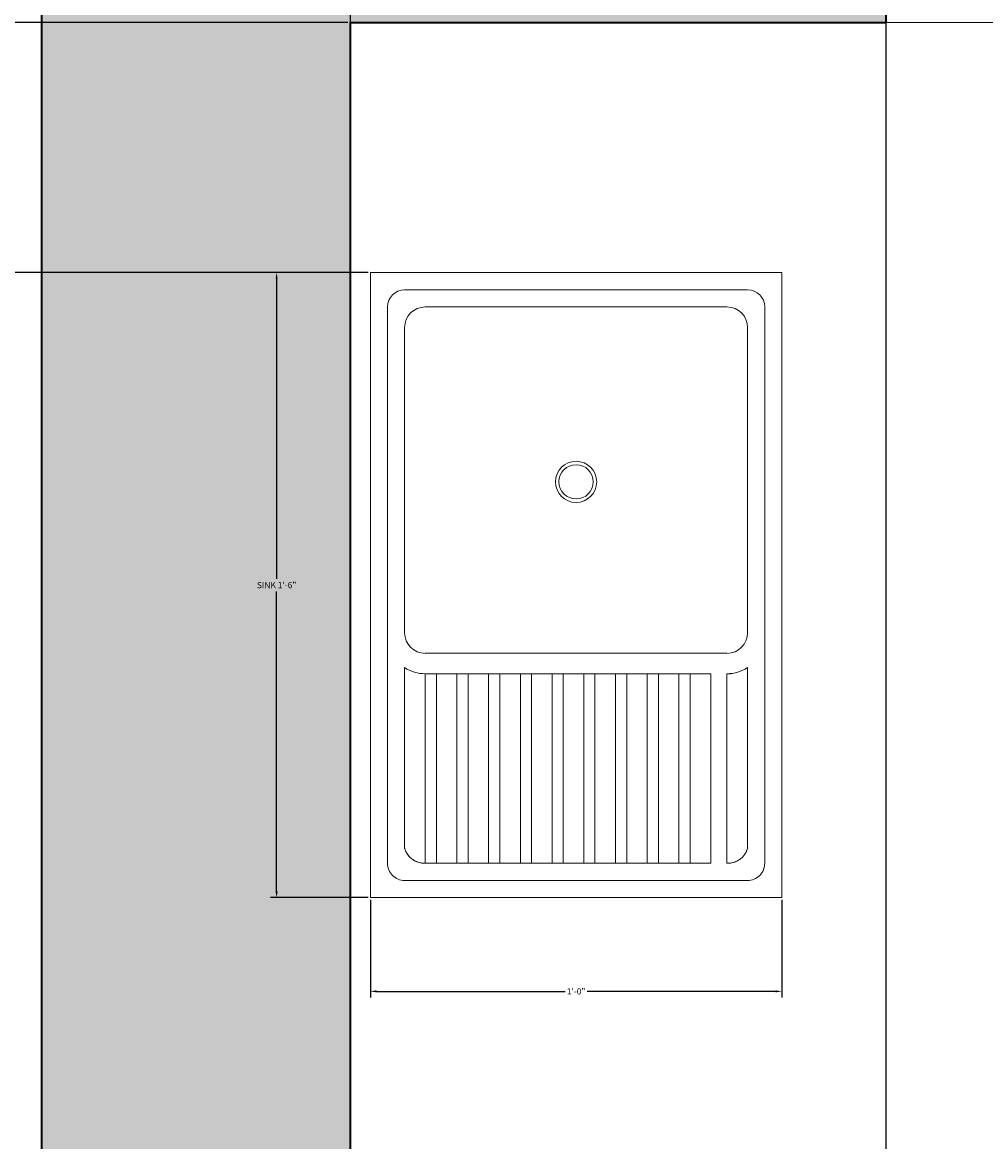
# Model space of a CAD drawing. Units: inches. Extents: x -5 to 330, y -522 to 40.
# Tile 10 of 23: x 23 to 51, y -330 to -297. Entities that reach past the tile are written whole.
import ezdxf

# ---------------------------------------------------------------- set-up
doc = ezdxf.new("R2010")
doc.units = ezdxf.units.IN
doc.header["$MEASUREMENT"] = 0
doc.linetypes.add('ACAD_ISO02W100', pattern=[15, 12, -3])
for name, color, linetype, lineweight in [('A-ANNO-DIMS', 2, 'Continuous', 18), ('A-FLOR-CASE', 8, 'Continuous', 25), ('A-FLOR-FIXT', 8, 'Continuous', 18), ('A-WALL', 7, 'Continuous', 35), ('A-WALL-OVHD', 8, 'ACAD_ISO02W100', 18)]:
    doc.layers.add(name, color=color, linetype=linetype, lineweight=lineweight)
doc.layers.add('A-WALL-PATT', color=18, linetype='Continuous', lineweight=13, true_color=0x000000)
doc.styles.get("Standard").update_dxf_attribs({"font": 'arial.ttf'})
doc.dimstyles.get("Standard").update_dxf_attribs({"dimtxt": 0.18, "dimasz": 0.18, "dimexe": 0.18, "dimexo": 0.0625, "dimgap": 0.09, "dimtad": 0, "dimtih": 1, "dimtoh": 1, "dimdec": 0, "dimzin": 0, "dimdsep": 46, "dimlunit": 3, "dimtxsty": 'Standard', "dimcen": 0.09, "dimadec": 0, "dimazin": 0, "dimtfac": 1, "dimtdec": 0, "dimtofl": 0, "dimtmove": 0, "dimatfit": 3, "dimfxl": 1, "dimtolj": 1, "dimtzin": 0, "dimarcsym": 0})

# ---------------------------------------------------------------- blocks, each defined once
blk = doc.blocks.new('*D2')
at = {"layer": 'A-ANNO-DIMS', "color": 0, "lineweight": -2, "transparency": 16777216}
for p, q in [((23.447, 12.356), (6.274, 12.356)), ((6.454, 12.176), (6.454, -203.738)), ((6.454, -425.964), (6.454, -210.049)), ((23.447, -426.144), (6.274, -426.144))]:
    blk.add_line(p, q, dxfattribs=at)
at = {"layer": 'A-ANNO-DIMS', "color": 0, "transparency": 16777216}
for points in [[(6.424, 12.176), (6.484, 12.176), (6.454, 12.356)], [(6.424, -425.964), (6.484, -425.964), (6.454, -426.144)]]:
    blk.add_solid(points, dxfattribs=at)
at = {"layer": 'Defpoints', "color": 0, "transparency": 16777216}
for p in [(23.51, 12.356), (6.454, -426.144), (23.51, -426.144)]:
    blk.add_point(p, dxfattribs=at)
at = {"layer": 'A-ANNO-DIMS', "color": 0, "transparency": 16777216, "insert": (6.454, -206.894), "char_height": 6, "attachment_point": 5}
blk.add_mtext('\\A1;36\'-7"', dxfattribs=at)
blk = doc.blocks.new('М12 540х820')
for p, q in [((0, 540), (-820, 540)), ((-820, 540), (-820, 0)), ((0, 0), (0, 540)), ((-45, 517.5), (-775, 517.5)), ((-797.5, 495), (-797.5, 45)), ((-347.5, 495), (-748, 495)), ((-301.7, 495), (-64.8, 495)), ((-22.5, 45), (-22.5, 495)), ((-293.7, 468), (-293.7, 472.5)), ((-775, 468), (-775, 72)), ((-320.5, 468), (-320.5, 72)), ((-293.7, 468), (-45, 468)), ((-45, 469.5), (-45, 468)), ((-293.7, 446.6), (-45, 446.6)), ((-293.7, 419.6), (-293.7, 446.6)), ((-45, 419.6), (-45, 446.6)), ((-293.7, 419.6), (-45, 419.6)), ((-293.7, 405), (-45, 405)), ((-293.7, 378), (-293.7, 405)), ((-45, 378), (-45, 405)), ((-293.7, 378), (-45, 378)), ((-293.7, 336.4), (-293.7, 363.4)), ((-293.7, 363.4), (-45, 363.4)), ((-45, 336.4), (-45, 363.4)), ((-293.7, 336.4), (-45, 336.4)), ((-293.7, 294.7), (-293.7, 321.7)), ((-293.7, 321.7), (-45, 321.7)), ((-45, 294.7), (-45, 321.7)), ((-293.7, 294.7), (-45, 294.7)), ((-293.7, 253.1), (-293.7, 280.1)), ((-293.7, 280.1), (-45, 280.1)), ((-45, 253.1), (-45, 280.1)), ((-293.7, 253.1), (-45, 253.1)), ((-293.7, 211.5), (-293.7, 238.5)), ((-293.7, 238.5), (-45, 238.5)), ((-45, 211.5), (-45, 238.5)), ((-293.7, 211.5), (-45, 211.5)), ((-293.7, 169.9), (-293.7, 196.9)), ((-293.7, 196.9), (-45, 196.9)), ((-45, 169.9), (-45, 196.9)), ((-293.7, 169.9), (-45, 169.9)), ((-293.7, 128.2), (-293.7, 155.2)), ((-293.7, 155.2), (-45, 155.2)), ((-45, 128.2), (-45, 155.2)), ((-293.7, 128.2), (-45, 128.2)), ((-293.7, 113.6), (-45, 113.6)), ((-293.7, 86.6), (-293.7, 113.6)), ((-45, 86.6), (-45, 113.6)), ((-293.7, 86.6), (-45, 86.6)), ((-293.7, 72), (-45, 72)), ((-45, 70.5), (-45, 72)), ((-748, 45), (-347.5, 45)), ((-301.7, 45), (-64.8, 45)), ((-775, 22.5), (-45, 22.5)), ((-820, 0), (0, 0))]:
    blk.add_line(p, q)
at = {"ltscale": 0.06}
for p, q in [((-820, 0), (-820, 540)), ((-820, 540), (0, 540)), ((0, 540), (0, 536.9)), ((0, 536.9), (0, 0)), ((-293.7, 446.6), (-45, 446.6)), ((-293.7, 405), (-293.7, 446.6)), ((-45, 446.6), (-45, 419.6)), ((-45, 419.6), (-45, 378)), ((-293.7, 363.4), (-293.7, 405)), ((-45, 378), (-45, 336.4)), ((-293.7, 321.7), (-293.7, 363.4)), ((-45, 336.4), (-45, 294.7)), ((-293.7, 280.1), (-293.7, 321.7)), ((-45, 294.7), (-45, 253.1)), ((-293.7, 238.5), (-293.7, 280.1)), ((-45, 253.1), (-45, 211.5)), ((-293.7, 196.9), (-293.7, 238.5)), ((-45, 211.5), (-45, 169.9)), ((-293.7, 155.2), (-293.7, 196.9)), ((-45, 169.9), (-45, 128.2)), ((-293.7, 113.6), (-293.7, 155.2)), ((-45, 128.2), (-45, 86.6)), ((-293.7, 72), (-293.7, 113.6)), ((-45, 86.6), (-45, 72)), ((-45, 72), (-293.7, 72)), ((0, 0), (-820, 0))]:
    blk.add_line(p, q, dxfattribs=at)
at = {"extrusion": (0, 0, -1)}
for centre, major_axis, start_param, end_param in [((-775, 495), (-15.9, 15.9), -0.785398, 0.785398), ((-775, 495), (-15.9, 15.9), -0.785398, 0.785398), ((-45, 495), (-15.9, -15.9), 2.356194, 3.926991), ((-45, 495), (-15.9, -15.9), 2.356194, 3.926991), ((-748, 468), (-19.1, -19.1), 0.785398, 2.356194), ((-748, 468), (-19.1, -19.1), 0.785398, 2.356194), ((-347.5, 468), (-19.1, 19.1), 0.785398, 2.356194), ((-347.5, 468), (-19.1, 19.1), 0.785398, 2.356194), ((-343.2, 468), (-35, 35), 1.779263, 2.356194), ((-343.2, 468), (-35, 35), 1.779263, 2.356192), ((-72.3, 468.8), (-19.3, 19.3), 1.0328, 2.38382), ((-72.3, 468.8), (-19.3, 19.3), 1.0328, 1.064673), ((-72.3, 468.8), (-19.3, 19.3), 1.064673, 2.328569), ((-343.2, 468), (-35, 35), 2.356192, 2.356194), ((-72.3, 468.8), (-19.3, 19.3), 2.328569, 2.38382), ((-545.5, 270), (-19.1, -19.1), 3.926991, 10.210176), ((-545.5, 270), (-19.1, -19.1), 3.926991, 10.210176), ((-545.5, 270), (-15.9, -15.9), 3.926991, 10.210176), ((-545.5, 270), (-15.9, -15.9), 3.926991, 10.210176), ((-748, 72), (-19.1, 19.1), 3.926991, 5.497787), ((-748, 72), (-19.1, 19.1), 3.926991, 5.497787), ((-347.5, 72), (-19.1, -19.1), 3.926991, 5.497787), ((-347.5, 72), (-19.1, -19.1), 3.926991, 5.497787), ((-343.2, 72), (-35, -35), 3.926991, 4.503922), ((-343.2, 72), (-35, -35), 3.926991, 4.503922), ((-72.3, 71.2), (-19.3, -19.3), 3.899365, 5.250385), ((-72.3, 71.2), (-19.3, -19.3), 3.954617, 5.218512), ((-72.3, 71.2), (-19.3, -19.3), 3.899365, 3.954617), ((-775, 45), (-15.9, -15.9), 5.497787, 7.068583), ((-775, 45), (-15.9, -15.9), 5.497787, 7.068583), ((-72.3, 71.2), (-19.3, -19.3), 5.218512, 5.250385), ((-45, 45), (-15.9, 15.9), 2.356194, 3.926991), ((-45, 45), (-15.9, 15.9), 2.356194, 3.926991)]:
    blk.add_ellipse(centre, major_axis=major_axis, ratio=1, start_param=start_param, end_param=end_param, dxfattribs=at)
blk = doc.blocks.new('*D33')
at = {"layer": 'A-ANNO-DIMS', "color": 0, "lineweight": -2, "transparency": 16777216}
for p, q in [((33.036, -304.441), (30.185, -304.441)), ((30.365, -304.621), (30.365, -313.37)), ((30.365, -322.485), (30.365, -313.736)), ((33.036, -322.665), (30.185, -322.665))]:
    blk.add_line(p, q, dxfattribs=at)
at = {"layer": 'A-ANNO-DIMS', "color": 0, "transparency": 16777216}
for points in [[(30.335, -304.621), (30.395, -304.621), (30.365, -304.441)], [(30.335, -322.485), (30.395, -322.485), (30.365, -322.665)]]:
    blk.add_solid(points, dxfattribs=at)
at = {"layer": 'Defpoints', "color": 0, "transparency": 16777216}
for p in [(33.099, -304.441), (30.365, -322.665), (33.099, -322.665)]:
    blk.add_point(p, dxfattribs=at)
at = {"layer": 'A-ANNO-DIMS', "color": 0, "transparency": 16777216, "insert": (30.365, -313.553), "char_height": 0.18, "attachment_point": 5}
blk.add_mtext('\\A1;SINK 1\'-6"', dxfattribs=at)
blk = doc.blocks.new('*D34')
at = {"layer": 'A-ANNO-DIMS', "color": 0, "lineweight": -2, "transparency": 16777216}
for p, q in [((33.099, -322.728), (33.099, -325.579)), ((45.1, -322.728), (45.1, -325.579)), ((33.279, -325.399), (38.778, -325.399)), ((44.92, -325.399), (39.42, -325.399))]:
    blk.add_line(p, q, dxfattribs=at)
at = {"layer": 'A-ANNO-DIMS', "color": 0, "transparency": 16777216}
for points in [[(33.279, -325.369), (33.279, -325.429), (33.099, -325.399)], [(44.92, -325.369), (44.92, -325.429), (45.1, -325.399)]]:
    blk.add_solid(points, dxfattribs=at)
at = {"layer": 'Defpoints', "color": 0, "transparency": 16777216}
for p in [(33.099, -322.665), (45.1, -322.665), (45.1, -325.399)]:
    blk.add_point(p, dxfattribs=at)
at = {"layer": 'A-ANNO-DIMS', "color": 0, "transparency": 16777216, "insert": (39.099, -325.399), "char_height": 0.18, "attachment_point": 5}
blk.add_mtext('\\A1;1\'-0"', dxfattribs=at)
blk = doc.blocks.new('*D40')
at = {"layer": 'A-ANNO-DIMS', "color": 0, "lineweight": -2, "transparency": 16777216}
for p, q in [((32.51, -246.706), (32.51, -522.309)), ((79.01, -246.706), (79.01, -522.309)), ((32.69, -522.129), (55.151, -522.129)), ((78.83, -522.129), (56.369, -522.129))]:
    blk.add_line(p, q, dxfattribs=at)
at = {"layer": 'A-ANNO-DIMS', "color": 0, "transparency": 16777216}
for points in [[(32.69, -522.099), (32.69, -522.159), (32.51, -522.129)], [(78.83, -522.099), (78.83, -522.159), (79.01, -522.129)]]:
    blk.add_solid(points, dxfattribs=at)
at = {"layer": 'Defpoints', "color": 0, "transparency": 16777216}
for p in [(32.51, -246.644), (79.01, -246.644), (79.01, -522.129)]:
    blk.add_point(p, dxfattribs=at)
at = {"layer": 'A-ANNO-DIMS', "color": 0, "transparency": 16777216, "insert": (55.76, -522.129), "char_height": 0.18, "attachment_point": 5}
blk.add_mtext('\\A1;3\'-10 1/2"', dxfattribs=at)
blk = doc.blocks.new('*D47')
at = {"layer": 'A-ANNO-DIMS', "color": 0, "lineweight": -2, "transparency": 16777216}
for p, q in [((32.447, -297.144), (-3.655, -297.144)), ((-3.475, -297.324), (-3.475, -300.609)), ((-3.475, -304.261), (-3.475, -300.975)), ((33.036, -304.441), (-3.655, -304.441))]:
    blk.add_line(p, q, dxfattribs=at)
at = {"layer": 'A-ANNO-DIMS', "color": 0, "transparency": 16777216}
for points in [[(-3.505, -297.324), (-3.445, -297.324), (-3.475, -297.144)], [(-3.505, -304.261), (-3.445, -304.261), (-3.475, -304.441)]]:
    blk.add_solid(points, dxfattribs=at)
at = {"layer": 'Defpoints', "color": 0, "transparency": 16777216}
for p in [(32.51, -297.144), (-3.475, -304.441), (33.099, -304.441)]:
    blk.add_point(p, dxfattribs=at)
at = {"layer": 'A-ANNO-DIMS', "color": 0, "transparency": 16777216, "insert": (-3.475, -300.792), "char_height": 0.18, "attachment_point": 5}
blk.add_mtext('\\A1;0\'-7 1/2"', dxfattribs=at)

msp = doc.modelspace()

# ---------------------------------------------------------------- hatches: boundary and pattern name
at = {"layer": 'A-WALL-PATT'}
h = msp.add_hatch(color=256, dxfattribs=at)
h.dxf.hatch_style = 1
h.paths.add_polyline_path([(164.01, -44.152), (159.51, -44.152), (159.51, -153.144), (164.01, -153.144)], flags=17)
h.paths.add_polyline_path([(224.01, -188.144), (272.01, -188.144), (272.01, -218.144), (260.01, -218.144), (260.01, -222.644), (272.01, -222.644), (272.01, -292.644), (159.01, -292.644), (159.01, -297.144), (272.01, -297.144), (272.01, -417.144), (245.51, -417.144), (245.51, -426.144), (272.01, -426.144), (272.01, -495.144), (281.01, -495.144), (281.01, 12.356), (23.51, 12.356), (23.51, -426.144), (62.918, -426.144), (62.918, -417.144), (32.51, -417.144), (32.51, -297.144), (48.129, -297.144), (48.129, -292.644), (32.51, -292.644), (32.51, -140.644), (133.51, -140.644), (133.51, -131.644), (32.51, -131.644), (32.51, 3.356), (159.51, 3.356), (164.01, 3.356), (220.01, 3.356), (224.51, 3.356), (272.01, 3.356), (272.01, -179.144), (159.51, -179.144), (159.51, -188.144), (219.51, -188.144), (219.51, -266.644), (224.01, -266.644), (224.01, -222.644), (236.01, -222.644), (236.01, -218.144), (224.01, -218.144)])
h.paths.add_polyline_path([(133.01, -292.644), (128.51, -292.644), (128.51, -297.144), (128.51, -417.144), (122.918, -417.144), (122.918, -426.144), (133.01, -426.144)], flags=17)
h.paths.add_polyline_path([(185.51, -417.144), (159.01, -417.144), (159.01, -426.144), (185.51, -426.144)], flags=17)
h.paths.add_polyline_path([(133.51, -140.644), (129.01, -140.644), (129.01, -246.644), (133.51, -246.644)], flags=17)
h.paths.add_polyline_path([(246.01, -48.644), (224.51, -48.644), (224.51, -27.627), (220.01, -27.627), (220.01, -48.644), (198.604, -48.644), (198.604, -53.144), (246.01, -53.144)], flags=17)

# ---------------------------------------------------------------- linework, layer by layer
at = {"layer": 'A-FLOR-CASE'}
msp.add_line((48.129, -297.144), (48.129, -393.928), dxfattribs=at)
at = {"layer": 'A-WALL'}
for p, q in [((23.51, 12.356), (23.51, -495.144)), ((48.129, -292.644), (48.129, -297.144)), ((32.51, -297.144), (48.129, -297.144)), ((32.51, -297.144), (32.51, -417.144))]:
    msp.add_line(p, q, dxfattribs=at)
at = {"layer": 'A-WALL-OVHD'}
msp.add_line((48.129, -297.144), (128.51, -297.144), dxfattribs=at)

# ---------------------------------------------------------------- block references
at = {"layer": 'A-FLOR-FIXT', "xscale": 0.0222246795123264, "yscale": 0.0222246795123264, "zscale": 0.0222246795123264, "rotation": 270}
msp.add_blockref('М12 540х820', (33.099, -322.665), dxfattribs=at)

# ---------------------------------------------------------------- dimensions: what is measured, and where the dimension line sits
at = {"layer": 'A-ANNO-DIMS'}
for base, p1, p2, override, picture, middle in [((6.454321893, -426.143582029), (23.509888577, 12.356417971), (23.509888577, -426.143582029), {"dimtxt": 6, "dimclrd": 0, "dimclre": 0, "dimclrt": 0}, '*D2', (6.454321893, -206.893582029)), ((-3.475, -304.441), (32.51, -297.144), (33.099, -304.441), {"dimdec": 1, "dimlfac": 1, "dimrnd": 0, "dimzin": 1, "dimdsep": 46, "dimlunit": 4, "dimfrac": 2}, '*D47', (-3.475, -300.792))]:
    dim = msp.add_linear_dim(base=base, p1=p1, p2=p2, angle=90, dimstyle='Standard', override=override, dxfattribs=at)
    dim.commit()
    dim.dimension.update_dxf_attribs({"geometry": picture, "text_midpoint": middle})
for base, p1, p2, picture, middle in [((79.01, -522.129), (32.51, -246.644), (79.01, -246.644), '*D40', (55.76, -522.129)), ((45.1, -325.399), (33.099, -322.665), (45.1, -322.665), '*D34', (39.099, -325.399))]:
    dim = msp.add_linear_dim(base=base, p1=p1, p2=p2, dimstyle='Standard', override={"dimdec": 1, "dimlfac": 1, "dimrnd": 0, "dimzin": 1, "dimdsep": 46, "dimlunit": 4, "dimfrac": 2}, dxfattribs=at)
    dim.commit()
    dim.dimension.update_dxf_attribs({"geometry": picture, "text_midpoint": middle})
dim = msp.add_linear_dim(base=(30.365, -322.665), p1=(33.099, -304.441), p2=(33.099, -322.665), angle=270, text='SINK <>', dimstyle='Standard', override={"dimdec": 1, "dimlfac": 1, "dimrnd": 0, "dimzin": 1, "dimdsep": 46, "dimlunit": 4, "dimfrac": 2}, dxfattribs=at)
dim.commit()
dim.dimension.update_dxf_attribs({"geometry": '*D33', "text_midpoint": (30.365, -313.553)})

doc.saveas('drawing.dxf')
